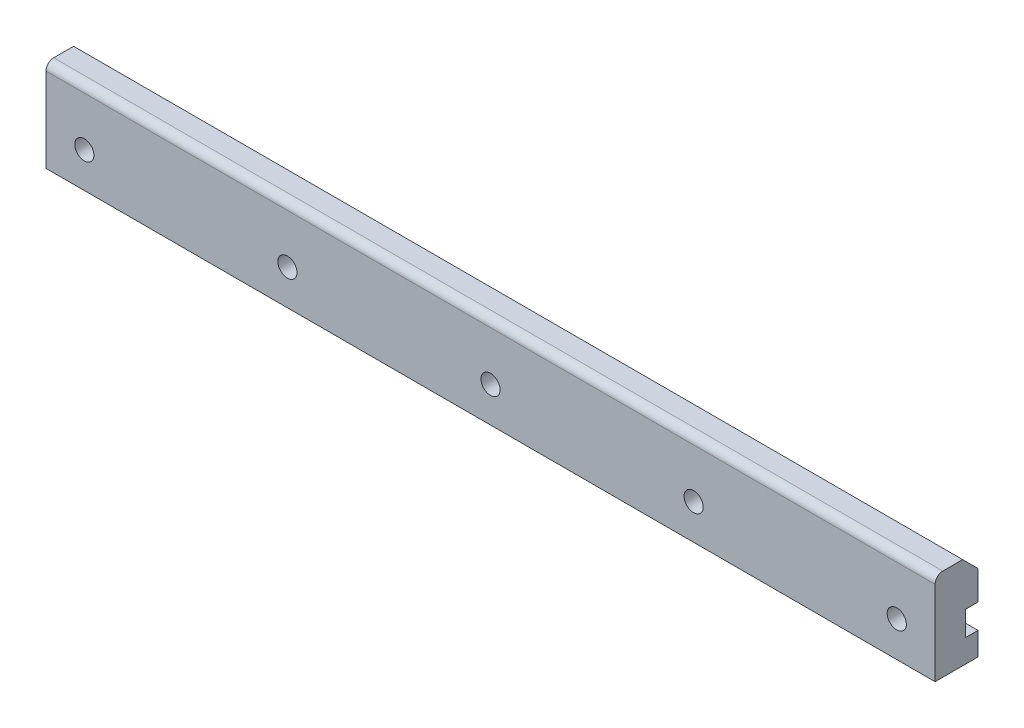
from build123d import *

# Parameters (mm, degrees)
RAIL_PROFILE_SKETCH_W           = 580
RAIL_PROFILE_SKETCH_H           = 60
RAIL_BAR_580X60X28_DEPTH        = 28
EDGE_FILLET_R5_R                = 5
GROOVE_SKETCH_W                 = 16
GROOVE_SKETCH_H                 = 16
LONGITUDINAL_GROOVE_16X16_DEPTH = 582.449911858
EDGE_CHAMFER_10X45_SIZE         = 10
MOUNTING_HOLES_SKETCH_R         = 6.25
MOUNTING_HOLES_5X_DEPTH         = 293.889057494


with BuildPart() as part:
    # Rail Profile Sketch → Rail Bar 580x60x28 (new body)
    with BuildSketch(Plane.XY):
        Rectangle(RAIL_PROFILE_SKETCH_W, RAIL_PROFILE_SKETCH_H)
    extrude(amount=RAIL_BAR_580X60X28_DEPTH)

    # Edge Fillet R5
    edge_fillet_r5_edges = [part.edges().sort_by_distance(p)[0] for p in [
        (0, 30, 28),
    ]]
    fillet(edge_fillet_r5_edges, radius=EDGE_FILLET_R5_R)

    # Groove Sketch → Longitudinal Groove 16x16 (cut, through all)
    with BuildSketch(Plane(origin=(290, 0, 0), x_dir=(0, 0, -1), z_dir=(1, 0, 0))):
        with Locations((0, -7)):
            Rectangle(GROOVE_SKETCH_W, GROOVE_SKETCH_H)
    extrude(amount=-LONGITUDINAL_GROOVE_16X16_DEPTH, mode=Mode.SUBTRACT)

    # Edge Chamfer 10x45
    edge_chamfer_10x45_edges = [part.edges().sort_by_distance(p)[0] for p in [
        (0, 30, 0),
    ]]
    chamfer(edge_chamfer_10x45_edges, length=EDGE_CHAMFER_10X45_SIZE)

    # Mounting Holes Sketch → Mounting Holes 5x (cut, through all)
    with BuildSketch(Plane.XY.offset(28)):
        with Locations((-265, -7)):
            Circle(MOUNTING_HOLES_SKETCH_R)
        with Locations((-132.5, -7)):
            Circle(MOUNTING_HOLES_SKETCH_R)
        with Locations((0, -7)):
            Circle(MOUNTING_HOLES_SKETCH_R)
        with Locations((132.5, -7)):
            Circle(MOUNTING_HOLES_SKETCH_R)
        with Locations((265, -7)):
            Circle(MOUNTING_HOLES_SKETCH_R)
    extrude(amount=-MOUNTING_HOLES_5X_DEPTH, mode=Mode.SUBTRACT)


solid = part.part
